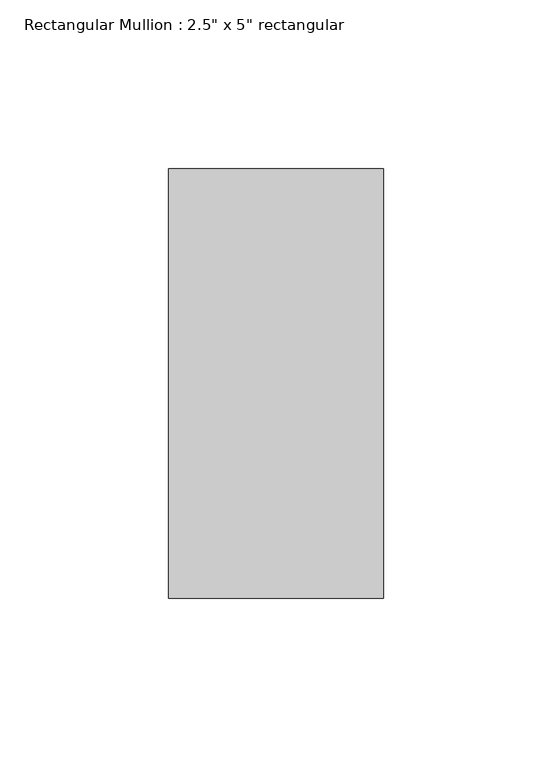
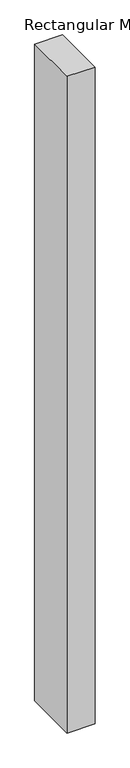
"""IFC4 building model written with IfcOpenShell, lengths in millimetres: member geometry."""

from ifc_helpers import new_model, si_unit, frame, origin, place, context, project, spatial, polyline, outline, extrude, source, transform, mapped, element, save


def member_2e0784aa(model_context):
    return source(origin(), model_context, "Body", "SweptSolid", [
        extrude(outline(polyline([(0.0, 63.5), (0.0, -63.5), (-63.5, -63.5), (-63.5, 63.5), (0.0, 63.5)])), frame((0.0, 0.0, -1571.3949481), z_axis=(0.0, 0.0, 1.0), x_axis=(1.0, 0.0, 0.0)), (0.0, 0.0, 1.0), 1571.3949481),
    ])


if __name__ == "__main__":
    model = new_model("IFC4")
    model_context = context("Model", 3, world=origin())
    ifc_project = project(units=[si_unit("LENGTHUNIT", "METRE", prefix="MILLI")], contexts=[model_context])
    site = spatial("IfcSite", under=ifc_project)
    building = spatial("IfcBuilding", under=site)
    placement = place(None, origin())
    member_shape = member_2e0784aa(model_context)
    element("IfcMember", 1, ObjectType="Rectangular Mullion : 2.5\" x 5\" rectangular", at=placement, inside=building, context=model_context, shape_type="MappedRepresentation", body=[
        mapped(member_shape, transform((0.0, 0.0, 0.0), x_axis=(1.0, 0.0, 0.0), y_axis=(0.0, 1.0, 0.0), z_axis=(0.0, 0.0, 1.0))),
    ])
    save(model, "model.ifc")

# Revit data of these elements
# Type "Rectangular Mullion : 2.5\" x 5\" rectangular"
#   built-in parameter 1007304 = 0.416667 (stored number, unit not read)
#   built-in parameter 1007301 = 0.104167 (stored number, unit not read)
#   built-in parameter 1007300 = 0.104167 (stored number, unit not read)
# Element 1 (IfcMember, "Rectangular Mullion : 2.5\" x 5\" rectangular")
#   Materials on its faces: "Aluminum"
# Materials
#   "Aluminum": class "Metal", colour RGB 247 247 247, transparency 0, Description = "Aluminum 6061", Cost = 0
